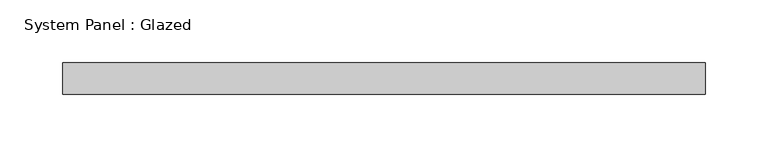
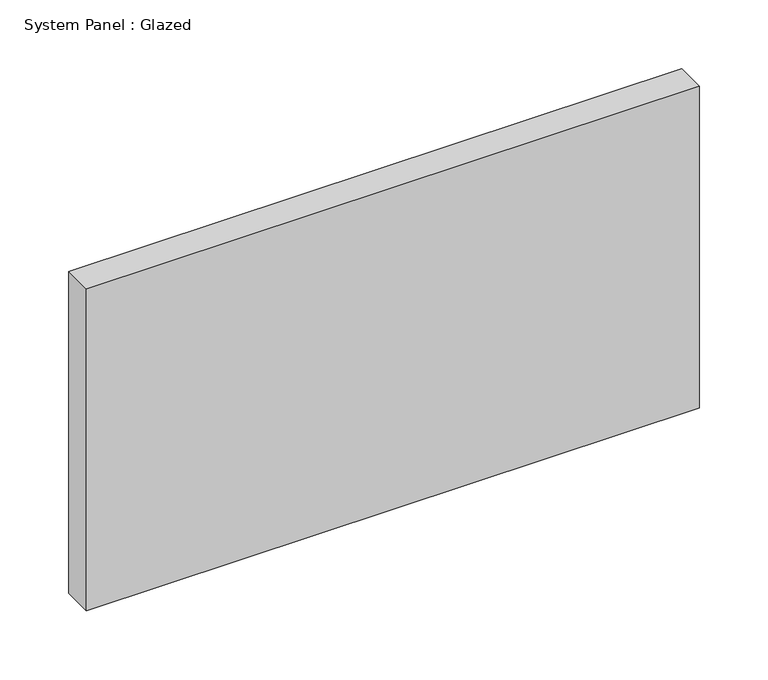
"""IFC4 building model written with IfcOpenShell, lengths in millimetres: plate geometry, System Panel : Glazed."""

from ifc_helpers import new_model, si_unit, origin, origin_with_axes, place, context, project, spatial, polyline, outline, extrude, source, transform, mapped, element, save


def system_panel_glazed_5422c98d(model_context):
    return source(origin(), model_context, "Body", "SweptSolid", [
        extrude(outline(polyline([(257.175, 19.05), (-257.175, 19.05), (-257.175, 44.45), (257.175, 44.45), (257.175, 19.05)])), origin_with_axes(), (0.0, 0.0, 1.0), 285.75),
    ])


if __name__ == "__main__":
    model = new_model("IFC4")
    model_context = context("Model", 3, world=origin())
    ifc_project = project(units=[si_unit("LENGTHUNIT", "METRE", prefix="MILLI")], contexts=[model_context])
    site = spatial("IfcSite", under=ifc_project)
    building = spatial("IfcBuilding", under=site)
    placement = place(None, origin())
    system_panel_glazed_shape = system_panel_glazed_5422c98d(model_context)
    element("IfcPlate", 1, ObjectType="System Panel : Glazed", at=placement, inside=building, context=model_context, shape_type="MappedRepresentation", body=[
        mapped(system_panel_glazed_shape, transform((0.0, 0.0, 0.0), x_axis=(1.0, 0.0, 0.0), y_axis=(0.0, 1.0, 0.0), z_axis=(0.0, 0.0, 1.0))),
    ])
    save(model, "model.ifc")

# Revit data of these elements
# Type "System Panel : Glazed"
#   Construction Type Id = "GSP4R"
#   Analytic Construction = "1/8 in Pilkington single glazing"
#   Visual Light Transmittance = 0.9
#   Solar Heat Gain Coefficient = 0.86
#   Heat Transfer Coefficient (U) = 1.18115 BTU/(h·ft²·°F)
#   Define Thermal Properties by = 1
# Element 1 (IfcPlate, "System Panel : Glazed")
#   Materials on its faces: "Glass"
# Materials
#   "Glass": class "Glass", colour RGB 0 128 192, transparency 0.75, Description = "Soda Lime Glass", Cost = 0
